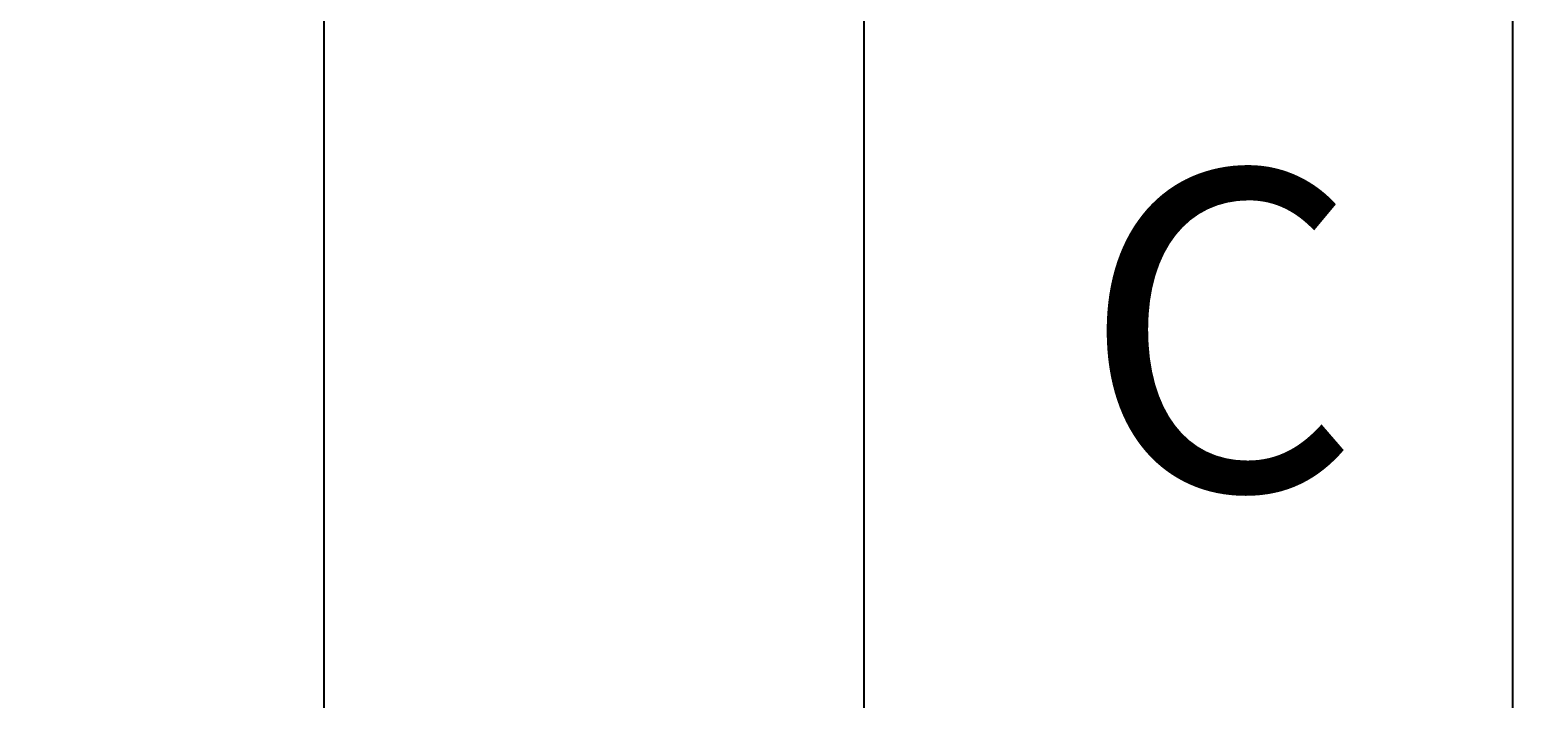
# Model space of a CAD drawing. Units: inches. Extents: x 35362 to 73946, y 43607 to 67532.
# Tile 89 of 134: x 51337 to 52380, y 48331 to 48793. Entities that reach past the tile are written whole.
import ezdxf

# ---------------------------------------------------------------- set-up
doc = ezdxf.new("R2010")
doc.units = ezdxf.units.IN
doc.header["$MEASUREMENT"] = 0
for name, color, linetype, lineweight in [('A-ANNO-DIMS', 2, 'Continuous', 18), ('E-ANNO-TEXT', 5, 'Continuous', 18), ('E-WIRE', 3, 'Continuous', 25)]:
    doc.layers.add(name, color=color, linetype=linetype, lineweight=lineweight)
doc.styles.get("Standard").update_dxf_attribs({"font": 'arial.ttf'})
doc.dimstyles.get("Standard").update_dxf_attribs({"dimtxt": 0.18, "dimasz": 0.18, "dimexe": 0.18, "dimexo": 0.0625, "dimgap": 0.09, "dimtad": 0, "dimtih": 1, "dimtoh": 1, "dimdec": 4, "dimzin": 0, "dimdsep": 46, "dimtxsty": 'Standard', "dimcen": 0.09, "dimadec": 0, "dimazin": 0, "dimtfac": 1, "dimtdec": 4, "dimtofl": 0, "dimtmove": 0, "dimatfit": 3, "dimfxl": 1, "dimtolj": 1, "dimtzin": 0, "dimarcsym": 0})

# ---------------------------------------------------------------- blocks, each defined once
blk = doc.blocks.new('*D11')
at = {"layer": 'A-ANNO-DIMS', "color": 0, "lineweight": -2, "transparency": 16777216}
for p, q in [((47978.7, 56028.8), (47978.7, 43606.7)), ((53109.8, 56028.8), (53109.8, 43606.7)), ((47978.8, 43606.9), (50543.9, 43606.9)), ((53109.6, 43606.9), (50544.6, 43606.9))]:
    blk.add_line(p, q, dxfattribs=at)
at = {"layer": 'A-ANNO-DIMS', "color": 0, "transparency": 16777216}
for points in [[(47978.8, 43606.9), (47978.8, 43606.8), (47978.7, 43606.9)], [(53109.6, 43606.9), (53109.6, 43606.8), (53109.8, 43606.9)]]:
    blk.add_solid(points, dxfattribs=at)
at = {"layer": 'Defpoints', "color": 0, "transparency": 16777216}
for p in [(47978.7, 56028.8), (53109.8, 56028.8), (53109.8, 43606.9)]:
    blk.add_point(p, dxfattribs=at)
at = {"layer": 'A-ANNO-DIMS', "color": 0, "transparency": 16777216, "insert": (50544.2, 43606.9), "char_height": 0.18, "attachment_point": 5}
blk.add_mtext('\\A1;5131', dxfattribs=at)
blk = doc.blocks.new('*D17')
at = {"layer": 'A-ANNO-DIMS', "color": 0, "lineweight": -2, "transparency": 16777216}
for p, q in [((49923.3, 61293.2), (49923.3, 43606.7)), ((51913.9, 61293.2), (51913.9, 43606.7)), ((49923.5, 43606.9), (50918.2, 43606.9)), ((51913.8, 43606.9), (50919.1, 43606.9))]:
    blk.add_line(p, q, dxfattribs=at)
at = {"layer": 'A-ANNO-DIMS', "color": 0, "transparency": 16777216}
for points in [[(49923.5, 43606.9), (49923.5, 43606.8), (49923.3, 43606.9)], [(51913.8, 43606.9), (51913.8, 43606.8), (51913.9, 43606.9)]]:
    blk.add_solid(points, dxfattribs=at)
at = {"layer": 'Defpoints', "color": 0, "transparency": 16777216}
for p in [(49923.3, 61293.3), (51913.9, 61293.3), (51913.9, 43606.9)]:
    blk.add_point(p, dxfattribs=at)
at = {"layer": 'A-ANNO-DIMS', "color": 0, "transparency": 16777216, "insert": (50918.6, 43606.9), "char_height": 0.18, "attachment_point": 5}
blk.add_mtext('\\A1;1990.6', dxfattribs=at)
blk = doc.blocks.new('*D67')
at = {"layer": 'A-ANNO-DIMS', "color": 0, "lineweight": -2, "transparency": 16777216}
for p, q in [((56873.5, 53351.5), (35361.8, 53351.5)), ((35361.9, 53351.3), (35361.9, 49400.9)), ((35361.9, 45450.1), (35361.9, 49400.5)), ((53793.6, 45449.9), (35361.8, 45449.9))]:
    blk.add_line(p, q, dxfattribs=at)
at = {"layer": 'A-ANNO-DIMS', "color": 0, "transparency": 16777216}
for points in [[(35361.9, 53351.3), (35362, 53351.3), (35361.9, 53351.5)], [(35361.9, 45450.1), (35362, 45450.1), (35361.9, 45449.9)]]:
    blk.add_solid(points, dxfattribs=at)
at = {"layer": 'Defpoints', "color": 0, "transparency": 16777216}
for p in [(35361.9, 53351.5), (56873.6, 53351.5), (53793.6, 45449.9)]:
    blk.add_point(p, dxfattribs=at)
at = {"layer": 'A-ANNO-DIMS', "color": 0, "transparency": 16777216, "insert": (35361.9, 49400.7), "char_height": 0.18, "attachment_point": 5}
blk.add_mtext('\\A1;7901.6', dxfattribs=at)
blk = doc.blocks.new('*D88')
at = {"layer": 'A-ANNO-DIMS', "color": 0, "lineweight": -2, "transparency": 16777216}
for p, q in [((52362.6, 48318.3), (52362.6, 67531.7)), ((52362.7, 67531.5), (52432.1, 67531.5)), ((52502.2, 67531.5), (52432.8, 67531.5)), ((52502.4, 48318.3), (52502.4, 67531.7))]:
    blk.add_line(p, q, dxfattribs=at)
at = {"layer": 'A-ANNO-DIMS', "color": 0, "transparency": 16777216}
for points in [[(52362.7, 67531.5), (52362.7, 67531.5), (52362.6, 67531.5)], [(52502.2, 67531.5), (52502.2, 67531.5), (52502.4, 67531.5)]]:
    blk.add_solid(points, dxfattribs=at)
at = {"layer": 'Defpoints', "color": 0, "transparency": 16777216}
for p in [(52502.4, 67531.5), (52362.6, 48318.3), (52502.4, 48318.3)]:
    blk.add_point(p, dxfattribs=at)
at = {"layer": 'A-ANNO-DIMS', "color": 0, "transparency": 16777216, "insert": (52432.5, 67531.5), "char_height": 0.18, "attachment_point": 5}
blk.add_mtext('\\A1;139.8', dxfattribs=at)
blk = doc.blocks.new('*D89')
at = {"layer": 'A-ANNO-DIMS', "color": 0, "lineweight": -2, "transparency": 16777216}
for p, q in [((53707.7, 48897.7), (35361.8, 48897.7)), ((35361.9, 48897.6), (35361.9, 48303.2)), ((35361.9, 47708.4), (35361.9, 48302.8)), ((53707.7, 47708.2), (35361.8, 47708.2))]:
    blk.add_line(p, q, dxfattribs=at)
at = {"layer": 'A-ANNO-DIMS', "color": 0, "transparency": 16777216}
for points in [[(35361.9, 48897.6), (35362, 48897.6), (35361.9, 48897.7)], [(35361.9, 47708.4), (35362, 47708.4), (35361.9, 47708.2)]]:
    blk.add_solid(points, dxfattribs=at)
at = {"layer": 'Defpoints', "color": 0, "transparency": 16777216}
for p in [(53707.8, 48897.7), (35361.9, 47708.2), (53707.8, 47708.2)]:
    blk.add_point(p, dxfattribs=at)
at = {"layer": 'A-ANNO-DIMS', "color": 0, "transparency": 16777216, "insert": (35361.9, 48303), "char_height": 0.18, "attachment_point": 5}
blk.add_mtext('\\A1;1189.5', dxfattribs=at)

msp = doc.modelspace()

# ---------------------------------------------------------------- linework, layer by layer
at = {"layer": 'E-WIRE'}
msp.add_line((51540.551, 48956.924), (51540.551, 47918.089), dxfattribs=at)

# ---------------------------------------------------------------- texts
at = {"layer": 'E-ANNO-TEXT'}
msp.add_text('C', height=220.866, dxfattribs=at).set_placement((52064.339, 48475.033))

# ---------------------------------------------------------------- dimensions: what is measured, and where the dimension line sits
at = {"layer": 'A-ANNO-DIMS'}
for base, p1, p2, override, picture, middle in [((52502.363, 67531.512), (52362.557, 48318.269), (52502.363, 48318.269), {"dimdec": 1, "dimlfac": 1, "dimrnd": 0, "dimzin": 0, "dimdsep": 46, "dimlunit": 2}, '*D88', (52432.46, 67531.512)), ((51913.931, 43606.859), (49923.307, 61293.286), (51913.931, 61293.286), {"dimdec": 1, "dimlfac": 1, "dimrnd": 0, "dimzin": 0, "dimdsep": 46, "dimlunit": 2}, '*D17', (50918.619, 43606.859)), ((53109.76, 43606.859), (47978.665, 56028.836), (53109.76, 56028.836), {"dimdec": 0, "dimlfac": 1, "dimrnd": 0, "dimzin": 0, "dimdsep": 46, "dimlunit": 2}, '*D11', (50544.212, 43606.859))]:
    dim = msp.add_linear_dim(base=base, p1=p1, p2=p2, dimstyle='Standard', override=override, dxfattribs=at)
    dim.commit()
    dim.dimension.update_dxf_attribs({"geometry": picture, "text_midpoint": middle})
for base, p1, p2, picture, middle in [((35361.949, 53351.529), (53793.638, 45449.894), (56873.602, 53351.529), '*D67', (35361.949, 49400.712)), ((35361.949, 47708.216), (53707.781, 48897.738), (53707.781, 47708.216), '*D89', (35361.949, 48302.977))]:
    dim = msp.add_linear_dim(base=base, p1=p1, p2=p2, angle=90, dimstyle='Standard', override={"dimdec": 1, "dimlfac": 1, "dimrnd": 0, "dimzin": 0, "dimdsep": 46, "dimlunit": 2}, dxfattribs=at)
    dim.commit()
    dim.dimension.update_dxf_attribs({"geometry": picture, "text_midpoint": middle})

doc.saveas('drawing.dxf')
